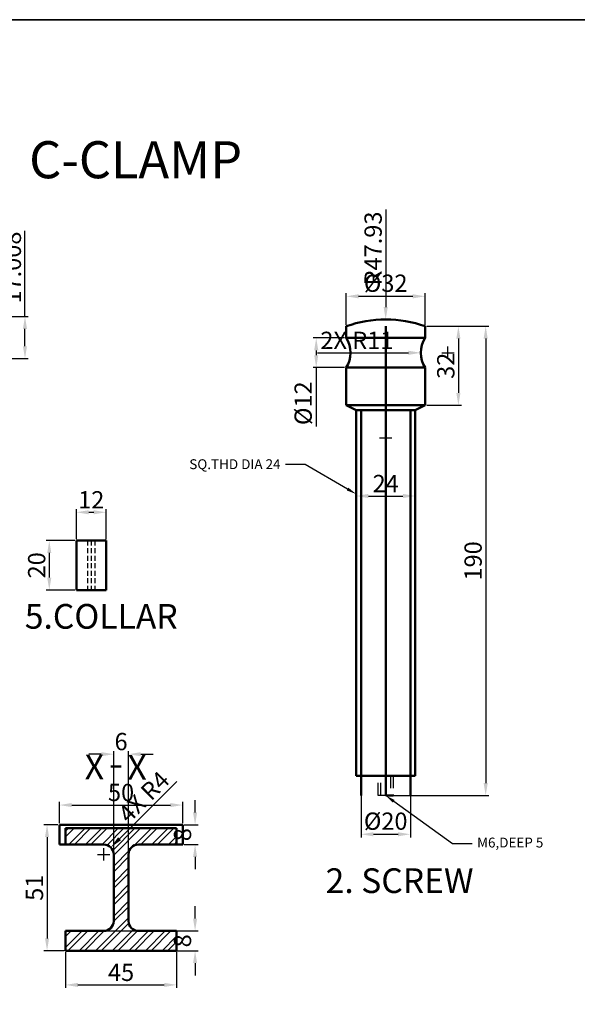
# Model space of a CAD drawing. Units: millimetres. Extents: x 210 to 1120, y -242 to 418.
# Tile 3 of 4: x 563 to 789, y 20 to 418. Entities that reach past the tile are written whole.
import ezdxf
from ezdxf import colors
from ezdxf.entities.mleader import LeaderData, LeaderLine
from ezdxf.math import Vec2, Vec3

# ---------------------------------------------------------------- set-up
doc = ezdxf.new("R2010")
doc.units = ezdxf.units.MM
doc.header["$LTSCALE"] = 0.4
doc.linetypes.add('DASHED', pattern=[19.05, 12.7, -6.35])
for name, color, linetype, lineweight in [('M-DIMS', 2, 'Continuous', 25), ('M-HATC', 8, 'Continuous', 18), ('M-HIDN', 4, 'DASHED', 25), ('M-OUTL', 7, 'Continuous', 50), ('M-TEXT', 3, 'Continuous', 25), ('M-TTLB', 7, 'Continuous', 35)]:
    doc.layers.add(name, color=color, linetype=linetype, lineweight=lineweight)
doc.styles.get("Standard").update_dxf_attribs({"font": 'arial.ttf'})
doc.dimstyles.new('ISO-25', dxfattribs={"dimtxt": 7, "dimasz": 5, "dimexe": 1.25, "dimexo": 0.625, "dimtad": 1, "dimtxsty": 'Standard', "dimcen": 2.5, "dimadec": 0, "dimazin": 0, "dimtfac": 1, "dimtofl": 0, "dimtmove": 0, "dimatfit": 3, "dimfxl": 1, "dimarcsym": 0})

# ---------------------------------------------------------------- blocks, each defined once
blk = doc.blocks.new('*D18')
at = {"layer": 'Defpoints', "color": 0, "transparency": 16777216}
for p in [(581.44, 41.35), (626.44, 41.35), (626.44, 27.51)]:
    blk.add_point(p, dxfattribs=at)
at = {"layer": 'M-DIMS', "color": 0, "lineweight": -2, "transparency": 16777216}
for p, q in [((581.44, 40.72), (581.44, 26.26)), ((626.44, 40.72), (626.44, 26.26)), ((586.44, 27.51), (621.44, 27.51))]:
    blk.add_line(p, q, dxfattribs=at)
at = {"layer": 'M-DIMS', "color": 0, "transparency": 16777216}
for points in [[(586.44, 28.34), (586.44, 26.67), (581.44, 27.51)], [(621.44, 28.34), (621.44, 26.67), (626.44, 27.51)]]:
    blk.add_solid(points, dxfattribs=at)
at = {"layer": 'M-DIMS', "color": 0, "transparency": 16777216, "insert": (603.94, 31.69), "char_height": 7, "attachment_point": 5}
blk.add_mtext('45', dxfattribs=at)
blk = doc.blocks.new('*D19')
at = {"layer": 'Defpoints', "color": 0, "transparency": 16777216}
for p in [(628.94, 100.33), (578.94, 92.35), (628.94, 92.35)]:
    blk.add_point(p, dxfattribs=at)
at = {"layer": 'M-DIMS', "color": 0, "lineweight": -2, "transparency": 16777216}
for p, q in [((578.94, 92.97), (578.94, 101.58)), ((583.94, 100.33), (623.94, 100.33)), ((628.94, 92.97), (628.94, 101.58))]:
    blk.add_line(p, q, dxfattribs=at)
at = {"layer": 'M-DIMS', "color": 0, "transparency": 16777216}
for points in [[(583.94, 101.17), (583.94, 99.5), (578.94, 100.33)], [(623.94, 101.17), (623.94, 99.5), (628.94, 100.33)]]:
    blk.add_solid(points, dxfattribs=at)
at = {"layer": 'M-DIMS', "color": 0, "transparency": 16777216, "insert": (603.94, 104.53), "char_height": 7, "attachment_point": 5}
blk.add_mtext('50', dxfattribs=at)
blk = doc.blocks.new('*D21')
at = {"layer": 'Defpoints', "color": 0, "transparency": 16777216}
for p in [(727.19, 306.33), (695.19, 294.2), (727.19, 294.2)]:
    blk.add_point(p, dxfattribs=at)
at = {"layer": 'M-DIMS', "color": 0, "lineweight": -2, "transparency": 16777216}
for p, q in [((695.19, 294.83), (695.19, 307.58)), ((727.19, 294.83), (727.19, 307.58)), ((700.19, 306.33), (722.19, 306.33))]:
    blk.add_line(p, q, dxfattribs=at)
at = {"layer": 'M-DIMS', "color": 0, "transparency": 16777216}
for points in [[(700.19, 307.17), (700.19, 305.5), (695.19, 306.33)], [(722.19, 307.17), (722.19, 305.5), (727.19, 306.33)]]:
    blk.add_solid(points, dxfattribs=at)
at = {"layer": 'M-DIMS', "color": 0, "transparency": 16777216, "insert": (711.19, 310.73), "char_height": 7, "attachment_point": 5}
blk.add_mtext('%%C32', dxfattribs=at)
blk = doc.blocks.new('*D22')
at = {"layer": 'Defpoints', "color": 0, "transparency": 16777216}
for p in [(695.19, 289.46), (683.04, 277.46), (695.19, 277.46)]:
    blk.add_point(p, dxfattribs=at)
at = {"layer": 'M-DIMS', "color": 0, "lineweight": -2, "transparency": 16777216}
for p, q in [((694.56, 289.46), (681.79, 289.46)), ((683.04, 284.46), (683.04, 282.46)), ((694.56, 277.46), (681.79, 277.46)), ((683.04, 277.46), (683.04, 253.64))]:
    blk.add_line(p, q, dxfattribs=at)
at = {"layer": 'M-DIMS', "color": 0, "transparency": 16777216}
for points in [[(682.21, 284.46), (683.88, 284.46), (683.04, 289.46)], [(682.21, 282.46), (683.88, 282.46), (683.04, 277.46)]]:
    blk.add_solid(points, dxfattribs=at)
at = {"layer": 'M-DIMS', "color": 0, "transparency": 16777216, "insert": (678.65, 263.05), "char_height": 7, "attachment_point": 5, "rotation": 90}
blk.add_mtext('%%C12', dxfattribs=at)
blk = doc.blocks.new('*D23')
at = {"layer": 'Defpoints', "color": 0, "transparency": 16777216}
for p in [(727.19, 294.2), (727.19, 262.2), (740.65, 262.2)]:
    blk.add_point(p, dxfattribs=at)
at = {"layer": 'M-DIMS', "color": 0, "lineweight": -2, "transparency": 16777216}
for p, q in [((727.81, 294.2), (741.9, 294.2)), ((740.65, 289.2), (740.65, 267.2)), ((727.81, 262.2), (741.9, 262.2))]:
    blk.add_line(p, q, dxfattribs=at)
at = {"layer": 'M-DIMS', "color": 0, "transparency": 16777216}
for points in [[(739.82, 289.2), (741.48, 289.2), (740.65, 294.2)], [(739.82, 267.2), (741.48, 267.2), (740.65, 262.2)]]:
    blk.add_solid(points, dxfattribs=at)
at = {"layer": 'M-DIMS', "color": 0, "transparency": 16777216, "insert": (736.45, 278.2), "char_height": 7, "attachment_point": 5, "rotation": 90}
blk.add_mtext('32', dxfattribs=at)
blk = doc.blocks.new('*D24')
at = {"layer": 'Defpoints', "color": 0, "transparency": 16777216}
for p in [(701.19, 112.2), (721.19, 112.2), (721.19, 88.5)]:
    blk.add_point(p, dxfattribs=at)
at = {"layer": 'M-DIMS', "color": 0, "lineweight": -2, "transparency": 16777216}
for p, q in [((701.19, 111.58), (701.19, 87.25)), ((721.19, 111.58), (721.19, 87.25)), ((706.19, 88.5), (716.19, 88.5))]:
    blk.add_line(p, q, dxfattribs=at)
at = {"layer": 'M-DIMS', "color": 0, "transparency": 16777216}
for points in [[(706.19, 89.33), (706.19, 87.67), (701.19, 88.5)], [(716.19, 89.33), (716.19, 87.67), (721.19, 88.5)]]:
    blk.add_solid(points, dxfattribs=at)
at = {"layer": 'M-DIMS', "color": 0, "transparency": 16777216, "insert": (711.19, 92.9), "char_height": 7, "attachment_point": 5}
blk.add_mtext('%%C20', dxfattribs=at)
blk = doc.blocks.new('*D25')
at = {"layer": 'Defpoints', "color": 0, "ltscale": 0.4, "transparency": 16777216}
for p in [(699.19, 228.99), (723.19, 228.99), (723.19, 225.47)]:
    blk.add_point(p, dxfattribs=at)
at = {"layer": 'M-DIMS', "color": 0, "lineweight": -2, "ltscale": 0.4, "transparency": 16777216}
for p, q in [((699.19, 228.37), (699.19, 224.22)), ((723.19, 228.37), (723.19, 224.22)), ((704.19, 225.47), (718.19, 225.47))]:
    blk.add_line(p, q, dxfattribs=at)
at = {"layer": 'M-DIMS', "color": 0, "ltscale": 0.4, "transparency": 16777216}
for points in [[(704.19, 226.31), (704.19, 224.64), (699.19, 225.47)], [(718.19, 226.31), (718.19, 224.64), (723.19, 225.47)]]:
    blk.add_solid(points, dxfattribs=at)
at = {"layer": 'M-DIMS', "color": 0, "ltscale": 0.4, "transparency": 16777216, "insert": (711.19, 229.61), "char_height": 7, "attachment_point": 5}
blk.add_mtext('24', dxfattribs=at)
blk = doc.blocks.new('*D33')
at = {"layer": 'Defpoints', "color": 0, "ltscale": 0.4, "transparency": 16777216}
for p in [(727.19, 294.2), (711.19, 104.2), (751.72, 104.2)]:
    blk.add_point(p, dxfattribs=at)
at = {"layer": 'M-DIMS', "color": 0, "lineweight": -2, "ltscale": 0.4, "transparency": 16777216}
for p, q in [((727.81, 294.2), (752.97, 294.2)), ((751.72, 289.2), (751.72, 109.2)), ((711.81, 104.2), (752.97, 104.2))]:
    blk.add_line(p, q, dxfattribs=at)
at = {"layer": 'M-DIMS', "color": 0, "ltscale": 0.4, "transparency": 16777216}
for points in [[(750.88, 289.2), (752.55, 289.2), (751.72, 294.2)], [(750.88, 109.2), (752.55, 109.2), (751.72, 104.2)]]:
    blk.add_solid(points, dxfattribs=at)
at = {"layer": 'M-DIMS', "color": 0, "ltscale": 0.4, "transparency": 16777216, "insert": (747.52, 199.2), "char_height": 7, "attachment_point": 5, "rotation": 90}
blk.add_mtext('190', dxfattribs=at)
blk = doc.blocks.new('*D41')
at = {"layer": 'Defpoints', "color": 0, "ltscale": 0.4, "transparency": 16777216}
for p in [(597.86, 218.89), (585.86, 207.41), (597.86, 207.41)]:
    blk.add_point(p, dxfattribs=at)
at = {"layer": 'M-DIMS', "color": 0, "lineweight": -2, "ltscale": 0.4, "transparency": 16777216}
for p, q in [((585.86, 208.03), (585.86, 220.14)), ((597.86, 208.03), (597.86, 220.14)), ((590.86, 218.89), (592.86, 218.89))]:
    blk.add_line(p, q, dxfattribs=at)
at = {"layer": 'M-DIMS', "color": 0, "ltscale": 0.4, "transparency": 16777216}
for points in [[(590.86, 219.72), (590.86, 218.05), (585.86, 218.89)], [(592.86, 219.72), (592.86, 218.05), (597.86, 218.89)]]:
    blk.add_solid(points, dxfattribs=at)
at = {"layer": 'M-DIMS', "color": 0, "ltscale": 0.4, "transparency": 16777216, "insert": (591.86, 223.03), "char_height": 7, "attachment_point": 5}
blk.add_mtext('12', dxfattribs=at)
blk = doc.blocks.new('*D42')
at = {"layer": 'Defpoints', "color": 0, "ltscale": 0.4, "transparency": 16777216}
for p in [(585.86, 207.41), (574.84, 187.41), (585.86, 187.41)]:
    blk.add_point(p, dxfattribs=at)
at = {"layer": 'M-DIMS', "color": 0, "lineweight": -2, "ltscale": 0.4, "transparency": 16777216}
for p, q in [((585.24, 207.41), (573.59, 207.41)), ((574.84, 202.41), (574.84, 192.41)), ((585.24, 187.41), (573.59, 187.41))]:
    blk.add_line(p, q, dxfattribs=at)
at = {"layer": 'M-DIMS', "color": 0, "ltscale": 0.4, "transparency": 16777216}
for points in [[(574.01, 202.41), (575.67, 202.41), (574.84, 207.41)], [(574.01, 192.41), (575.67, 192.41), (574.84, 187.41)]]:
    blk.add_solid(points, dxfattribs=at)
at = {"layer": 'M-DIMS', "color": 0, "ltscale": 0.4, "transparency": 16777216, "insert": (570.64, 197.41), "char_height": 7, "attachment_point": 5, "rotation": 90}
blk.add_mtext('20', dxfattribs=at)
blk = doc.blocks.new('*D48')
at = {"layer": 'Defpoints', "color": 0, "ltscale": 0.4, "transparency": 16777216}
for p in [(342.72, 298.14), (565, 298.14), (432.22, 281.13)]:
    blk.add_point(p, dxfattribs=at)
at = {"layer": 'M-DIMS', "color": 0, "lineweight": -2, "ltscale": 0.4, "transparency": 16777216}
for p, q in [((565, 298.14), (565, 332.81)), ((343.34, 298.14), (566.25, 298.14)), ((565, 286.13), (565, 293.14)), ((432.84, 281.13), (566.25, 281.13))]:
    blk.add_line(p, q, dxfattribs=at)
at = {"layer": 'M-DIMS', "color": 0, "ltscale": 0.4, "transparency": 16777216}
for points in [[(564.16, 293.14), (565.83, 293.14), (565, 298.14)], [(564.16, 286.13), (565.83, 286.13), (565, 281.13)]]:
    blk.add_solid(points, dxfattribs=at)
at = {"layer": 'M-DIMS', "color": 0, "ltscale": 0.4, "transparency": 16777216, "insert": (560.8, 317.98), "char_height": 7, "attachment_point": 5, "rotation": 90}
blk.add_mtext('17.008', dxfattribs=at)
blk = doc.blocks.new('*D50')
at = {"layer": 'Defpoints', "color": 0, "ltscale": 0.4, "transparency": 16777216}
for p in [(578.94, 92.35), (573.94, 41.35), (581.44, 41.35)]:
    blk.add_point(p, dxfattribs=at)
at = {"layer": 'M-DIMS', "color": 0, "lineweight": -2, "ltscale": 0.4, "transparency": 16777216}
for p, q in [((578.32, 92.35), (572.69, 92.35)), ((573.94, 87.35), (573.94, 46.35)), ((580.82, 41.35), (572.69, 41.35))]:
    blk.add_line(p, q, dxfattribs=at)
at = {"layer": 'M-DIMS', "color": 0, "ltscale": 0.4, "transparency": 16777216}
for points in [[(573.11, 87.35), (574.77, 87.35), (573.94, 92.35)], [(573.11, 46.35), (574.77, 46.35), (573.94, 41.35)]]:
    blk.add_solid(points, dxfattribs=at)
at = {"layer": 'M-DIMS', "color": 0, "ltscale": 0.4, "transparency": 16777216, "insert": (569.74, 66.85), "char_height": 7, "attachment_point": 5, "rotation": 90}
blk.add_mtext('51', dxfattribs=at)
blk = doc.blocks.new('*D51')
at = {"layer": 'Defpoints', "color": 0, "ltscale": 0.4, "transparency": 16777216}
for p in [(581.44, 49.35), (633.94, 49.35), (581.44, 41.35)]:
    blk.add_point(p, dxfattribs=at)
at = {"layer": 'M-DIMS', "color": 0, "lineweight": -2, "ltscale": 0.4, "transparency": 16777216}
for p, q in [((633.94, 54.35), (633.94, 59.35)), ((582.07, 49.35), (635.19, 49.35)), ((582.07, 41.35), (635.19, 41.35)), ((633.94, 36.35), (633.94, 31.35))]:
    blk.add_line(p, q, dxfattribs=at)
at = {"layer": 'M-DIMS', "color": 0, "ltscale": 0.4, "transparency": 16777216}
for points in [[(633.11, 54.35), (634.77, 54.35), (633.94, 49.35)], [(633.11, 36.35), (634.77, 36.35), (633.94, 41.35)]]:
    blk.add_solid(points, dxfattribs=at)
at = {"layer": 'M-DIMS', "color": 0, "ltscale": 0.4, "transparency": 16777216, "insert": (629.74, 45.35), "char_height": 7, "attachment_point": 5, "rotation": 90}
blk.add_mtext('8', dxfattribs=at)
blk = doc.blocks.new('*D52')
at = {"layer": 'Defpoints', "color": 0, "ltscale": 0.4, "transparency": 16777216}
for p in [(628.94, 92.35), (633.94, 92.35), (628.94, 84.35)]:
    blk.add_point(p, dxfattribs=at)
at = {"layer": 'M-DIMS', "color": 0, "lineweight": -2, "ltscale": 0.4, "transparency": 16777216}
for p, q in [((633.94, 97.35), (633.94, 102.35)), ((629.57, 92.35), (635.19, 92.35)), ((629.57, 84.35), (635.19, 84.35)), ((633.94, 79.35), (633.94, 74.35))]:
    blk.add_line(p, q, dxfattribs=at)
at = {"layer": 'M-DIMS', "color": 0, "ltscale": 0.4, "transparency": 16777216}
for points in [[(633.11, 97.35), (634.77, 97.35), (633.94, 92.35)], [(633.11, 79.35), (634.77, 79.35), (633.94, 84.35)]]:
    blk.add_solid(points, dxfattribs=at)
at = {"layer": 'M-DIMS', "color": 0, "ltscale": 0.4, "transparency": 16777216, "insert": (629.74, 88.35), "char_height": 7, "attachment_point": 5, "rotation": 90}
blk.add_mtext('8', dxfattribs=at)
blk = doc.blocks.new('*D53')
at = {"layer": 'Defpoints', "color": 0, "ltscale": 0.4, "transparency": 16777216}
for p in [(606.94, 120.93), (600.94, 80.35), (606.94, 80.35)]:
    blk.add_point(p, dxfattribs=at)
at = {"layer": 'M-DIMS', "color": 0, "lineweight": -2, "ltscale": 0.4, "transparency": 16777216}
for p, q in [((595.94, 120.93), (590.94, 120.93)), ((600.94, 80.97), (600.94, 122.18)), ((606.94, 80.97), (606.94, 122.18)), ((611.94, 120.93), (616.94, 120.93))]:
    blk.add_line(p, q, dxfattribs=at)
at = {"layer": 'M-DIMS', "color": 0, "ltscale": 0.4, "transparency": 16777216}
for points in [[(595.94, 121.76), (595.94, 120.09), (600.94, 120.93)], [(611.94, 121.76), (611.94, 120.09), (606.94, 120.93)]]:
    blk.add_solid(points, dxfattribs=at)
at = {"layer": 'M-DIMS', "color": 0, "ltscale": 0.4, "transparency": 16777216, "insert": (603.94, 125.13), "char_height": 7, "attachment_point": 5}
blk.add_mtext('6', dxfattribs=at)
blk = doc.blocks.new('*D57')
at = {"layer": 'Defpoints', "color": 0, "ltscale": 0.4, "transparency": 16777216}
for p in [(596.94, 80.35), (599.77, 83.17)]:
    blk.add_point(p, dxfattribs=at)
at = {"layer": 'M-DIMS', "color": 0, "lineweight": -2, "ltscale": 0.4, "transparency": 16777216}
for p, q in [((626.56, 109.89), (603.31, 86.7)), ((594.44, 80.35), (599.44, 80.35)), ((596.94, 77.85), (596.94, 82.85))]:
    blk.add_line(p, q, dxfattribs=at)
at = {"layer": 'M-DIMS', "color": 0, "ltscale": 0.4, "transparency": 16777216}
blk.add_solid([(602.73, 87.29), (603.9, 86.11), (599.77, 83.17)], dxfattribs=at)
at = {"layer": 'M-DIMS', "color": 0, "ltscale": 0.4, "transparency": 16777216, "insert": (613.79, 102.98), "char_height": 7, "attachment_point": 5, "rotation": 44.9182}
blk.add_mtext('4X R4', dxfattribs=at)
blk = doc.blocks.new('*D58')
at = {"layer": 'Defpoints', "color": 0, "ltscale": 0.4, "transparency": 16777216}
for p in [(711.19, 296.95), (711.19, 249.02)]:
    blk.add_point(p, dxfattribs=at)
at = {"layer": 'M-DIMS', "color": 0, "lineweight": -2, "ltscale": 0.4, "transparency": 16777216}
for p, q in [((711.19, 341.49), (711.19, 301.95)), ((711.19, 246.52), (711.19, 251.52)), ((708.69, 249.02), (713.69, 249.02))]:
    blk.add_line(p, q, dxfattribs=at)
at = {"layer": 'M-DIMS', "color": 0, "ltscale": 0.4, "transparency": 16777216}
blk.add_solid([(710.36, 301.95), (712.02, 301.95), (711.19, 296.95)], dxfattribs=at)
at = {"layer": 'M-DIMS', "color": 0, "ltscale": 0.4, "transparency": 16777216, "insert": (706.99, 325.71), "char_height": 7, "attachment_point": 5, "rotation": 89.9994}
blk.add_mtext('R47.93', dxfattribs=at)
blk = doc.blocks.new('*D59')
at = {"layer": 'Defpoints', "color": 0, "ltscale": 0.4, "transparency": 16777216}
for p in [(725.41, 283.46), (736.41, 283.46)]:
    blk.add_point(p, dxfattribs=at)
at = {"layer": 'M-DIMS', "color": 0, "lineweight": -2, "ltscale": 0.4, "transparency": 16777216}
for p, q in [((683.62, 283.46), (720.41, 283.46)), ((733.91, 283.46), (738.91, 283.46)), ((736.41, 280.96), (736.41, 285.96))]:
    blk.add_line(p, q, dxfattribs=at)
at = {"layer": 'M-DIMS', "color": 0, "ltscale": 0.4, "transparency": 16777216}
blk.add_solid([(720.41, 284.29), (720.41, 282.62), (725.41, 283.46)], dxfattribs=at)
at = {"layer": 'M-DIMS', "color": 0, "ltscale": 0.4, "transparency": 16777216, "insert": (699.52, 287.6), "char_height": 7, "attachment_point": 5, "rotation": 0.0011}
blk.add_mtext('2X R11', dxfattribs=at)

msp = doc.modelspace()

# ---------------------------------------------------------------- hatches: boundary and pattern name
at = {"layer": 'M-HATC'}
h = msp.add_hatch(dxfattribs=at)
h.set_pattern_fill('ANSI32', color=256, scale=0.5)
h.paths.add_polyline_path([(626.4411, 90.9516), (581.4411, 90.9516), (581.4411, 84.349), (596.9411, 84.349, -0.41421356), (600.9411, 80.349), (600.9411, 53.349, -0.41421356), (596.9411, 49.349), (581.4411, 49.349), (581.4411, 41.349), (626.4411, 41.349), (626.4411, 49.349), (610.9411, 49.349, -0.41421356), (606.9411, 53.349), (606.9411, 80.349, -0.41421356), (610.9411, 84.349), (626.4411, 84.349)])

# ---------------------------------------------------------------- linework, layer by layer
at = {"layer": 'M-HIDN', "ltscale": 0.4}
for p, q in [((590.362, 207.4059), (590.362, 187.4059)), ((591.862, 207.4059), (591.862, 187.4059)), ((593.362, 207.4059), (593.362, 187.4059))]:
    msp.add_line(p, q, dxfattribs=at)
at = {"layer": 'M-HIDN'}
for p, q in [((708.1885, 104.2017), (708.1885, 112.2017)), ((709.1885, 104.2017), (709.1885, 112.2017)), ((713.1885, 112.2017), (713.1885, 104.2017)), ((714.1885, 112.2017), (714.1885, 104.2017)), ((711.1885, 104.2017), (708.1885, 104.2017))]:
    msp.add_line(p, q, dxfattribs=at)
at = {"layer": 'M-OUTL'}
for p, q in [((695.1885, 289.4572), (695.1885, 294.2017)), ((711.1885, 294.2017), (711.1885, 104.2017)), ((727.1885, 294.2017), (727.1885, 289.4572)), ((695.1885, 289.4572), (727.1885, 289.4572)), ((695.1885, 262.2017), (695.1885, 277.4572)), ((695.1885, 277.4572), (727.1885, 277.4572)), ((727.1885, 277.4572), (727.1885, 262.2017)), ((695.1885, 262.2017), (727.1885, 262.2017)), ((695.1885, 262.2017), (699.1885, 260.2017)), ((699.1885, 260.2017), (699.1885, 112.2017)), ((701.1885, 260.2017), (701.1885, 104.2017)), ((721.1885, 260.2017), (721.1885, 104.2017)), ((727.1885, 262.2017), (723.1885, 260.2017)), ((723.1885, 260.2017), (723.1885, 112.2017)), ((601.3631, 115.9264), (599.8342, 115.9264)), ((599.8342, 115.9264), (603.9853, 115.9264)), ((723.1885, 112.2017), (699.1885, 112.2017)), ((714.1885, 104.2017), (711.1885, 104.2017)), ((578.9411, 92.349), (628.9411, 92.349)), ((578.9411, 84.349), (578.9411, 92.349)), ((628.9411, 92.349), (628.9411, 84.349)), ((581.4411, 90.9516), (626.4411, 90.9516)), ((581.4411, 84.349), (581.4411, 90.9516)), ((626.4411, 90.9516), (626.4411, 84.349)), ((596.9411, 84.349), (578.9411, 84.349)), ((628.9411, 84.349), (610.9411, 84.349)), ((600.9411, 80.349), (600.9411, 53.349)), ((606.9411, 80.349), (606.9411, 53.349)), ((581.4411, 49.349), (596.9411, 49.349)), ((581.4411, 41.349), (581.4411, 49.349)), ((610.9411, 49.349), (626.4411, 49.349)), ((626.4411, 49.349), (626.4411, 41.349)), ((626.4411, 41.349), (581.4411, 41.349)), ((581.4411, 41.349), (626.4411, 41.349))]:
    msp.add_line(p, q, dxfattribs=at)
at = {"layer": 'M-OUTL', "ltscale": 0.4}
for p, q in [((699.1885, 260.2017), (723.1885, 260.2017)), ((585.862, 207.4059), (597.862, 207.4059)), ((585.862, 187.4059), (585.862, 207.4059)), ((597.862, 207.4059), (597.862, 187.4059)), ((597.862, 187.4059), (585.862, 187.4059))]:
    msp.add_line(p, q, dxfattribs=at)
at = {"layer": 'M-OUTL'}
for centre, radius, start, end in [((711.1885, 249.0204), 47.9307, 70.499481, 109.500519), ((685.9696, 283.4572), 10.9994, 326.942366, 33.057634), ((736.4074, 283.4572), 10.9994, 146.942366, 213.057634), ((596.9411, 80.349), 4, 0, 90), ((610.9411, 80.349), 4, 90, 180), ((596.9411, 53.349), 4, 270, 0), ((610.9411, 53.349), 4, 180, 270)]:
    msp.add_arc(centre, radius, start, end, dxfattribs=at)
at = {"layer": 'M-TTLB', "ltscale": 0.4}
msp.add_lwpolyline([(210.1659, 418.3486), (1119.5264, 418.3486), (1119.5264, -242.3444), (210.1659, -242.3444)], close=True, dxfattribs=at)

# ---------------------------------------------------------------- texts
at = {"layer": 'M-TEXT', "ltscale": 0.4, "insert": (452.2266, 369.1481), "char_height": 15, "attachment_point": 1}
msp.add_mtext_dynamic_manual_height_columns('\\pxqc; C-CLAMP', width=310.631866, gutter_width=12.5, heights=[0], dxfattribs=at)
at = {"layer": 'M-TEXT', "attachment_point": 1}
for s, width, insert, char_height in [('\\pxqc;{\\H0.66667x;5.COLLAR} ', 102.502816, (544.6548, 181.7422), 15), ('X', 4.451993, (589.2112, 120.7711), 10), ('X', 4.451993, (606.5122, 120.6317), 10), ('\\pxqc;{\\H0.66667x;2. SCREW} ', 102.831898, (665.4087, 74.7214), 15)]:
    msp.add_mtext_dynamic_manual_height_columns(s, width=width, gutter_width=12.5, heights=[0], dxfattribs=dict(at, insert=insert, char_height=char_height))

# ---------------------------------------------------------------- dimensions: what is measured, and where the dimension line sits
at = {"layer": 'M-DIMS', "ltscale": 0.4}
dim = msp.add_radius_dim(center=(711.1885, 249.0204), mpoint=(711.189, 296.951), dimstyle='ISO-25', override={"dimdec": 2, "dimlfac": 1, "dimrnd": 0, "dimzin": 0, "dimdsep": 46, "dimlunit": 2}, dxfattribs=at)
dim.commit()
dim.dimension.update_dxf_attribs({"geometry": '*D58', "text_midpoint": (711.1893, 325.7094), "dimtype": 164})
for base, p1, p2, override, picture, middle in [((564.9982, 298.1425), (432.2189, 281.1344), (342.7189, 298.1425), {"dimdec": 3, "dimlfac": 1, "dimrnd": 0, "dimzin": 0, "dimdsep": 46, "dimlunit": 2}, '*D48', (560.7991, 317.9752)), ((751.7164, 104.2017), (727.1885, 294.2017), (711.1885, 104.2017), {"dimclrd": 0, "dimclre": 0, "dimclrt": 0}, '*D33', (747.5174, 199.2017)), ((574.8398, 187.4059), (585.862, 207.4059), (585.862, 187.4059), {"dimclrd": 0, "dimclre": 0, "dimclrt": 0}, '*D42', (570.6407, 197.4059)), ((633.9411, 92.349), (628.9411, 84.349), (628.9411, 92.349), {"dimdec": 0, "dimlfac": 1, "dimrnd": 0, "dimzin": 0, "dimdsep": 46, "dimlunit": 2}, '*D52', (629.7421, 88.349)), ((573.9411, 41.349), (578.9411, 92.349), (581.4411, 41.349), {"dimdec": 0, "dimlfac": 1, "dimrnd": 0, "dimzin": 0, "dimdsep": 46, "dimlunit": 2}, '*D50', (569.7421, 66.849)), ((633.9411, 49.349), (581.4411, 41.349), (581.4411, 49.349), {"dimdec": 0, "dimlfac": 1, "dimrnd": 0, "dimzin": 0, "dimdsep": 46, "dimlunit": 2}, '*D51', (629.7421, 45.349))]:
    dim = msp.add_linear_dim(base=base, p1=p1, p2=p2, angle=90, dimstyle='ISO-25', override=override, dxfattribs=at)
    dim.commit()
    dim.dimension.update_dxf_attribs({"geometry": picture, "text_midpoint": middle})
at = {"layer": 'M-DIMS'}
for base, p1, p2, picture, middle in [((727.1885, 306.3337), (695.1885, 294.2017), (727.1885, 294.2017), '*D21', (711.1885, 310.7285)), ((721.1885, 88.5008), (701.1885, 112.2017), (721.1885, 112.2017), '*D24', (711.1885, 92.8956))]:
    dim = msp.add_linear_dim(base=base, p1=p1, p2=p2, text='%%C<>', dimstyle='ISO-25', override={"dimclrd": 0, "dimclre": 0, "dimclrt": 0}, dxfattribs=at)
    dim.commit()
    dim.dimension.update_dxf_attribs({"geometry": picture, "text_midpoint": middle})
at = {"layer": 'M-DIMS', "ltscale": 0.4}
for center, mpoint, text, picture, middle in [((736.4074, 283.4572), (725.4079, 283.457), '2X <>', '*D59', (699.5151, 287.5982)), ((596.9411, 80.349), (599.7736, 83.1734), '4X <>', '*D57', (613.7945, 102.983))]:
    dim = msp.add_radius_dim(center=center, mpoint=mpoint, text=text, dimstyle='ISO-25', override={"dimdec": 0, "dimlfac": 1, "dimrnd": 0, "dimzin": 0, "dimdsep": 46, "dimlunit": 2}, dxfattribs=at)
    dim.commit()
    dim.dimension.update_dxf_attribs({"geometry": picture, "text_midpoint": middle})
at = {"layer": 'M-DIMS'}
dim = msp.add_linear_dim(base=(740.6513, 262.2017), p1=(727.1885, 294.2017), p2=(727.1885, 262.2017), angle=90, dimstyle='ISO-25', override={"dimclrd": 0, "dimclre": 0, "dimclrt": 0}, dxfattribs=at)
dim.commit()
dim.dimension.update_dxf_attribs({"geometry": '*D23', "text_midpoint": (736.4499, 278.2017)})
dim = msp.add_linear_dim(base=(683.0418, 277.4572), p1=(695.1885, 289.4572), p2=(695.1885, 277.4572), angle=90, text='%%C<>', dimstyle='ISO-25', override={"dimclrd": 0, "dimclre": 0, "dimclrt": 0}, dxfattribs=at)
dim.commit()
dim.dimension.update_dxf_attribs({"geometry": '*D22', "text_midpoint": (678.647, 263.0464)})
at = {"layer": 'M-DIMS', "ltscale": 0.4}
for base, p1, p2, override, picture, middle in [((723.1885, 225.4725), (699.1885, 228.9917), (723.1885, 228.9917), {"dimclrd": 0, "dimclre": 0, "dimclrt": 0}, '*D25', (711.1885, 229.6118)), ((597.862, 218.8863), (585.862, 207.4059), (597.862, 207.4059), {"dimclrd": 0, "dimclre": 0, "dimclrt": 0}, '*D41', (591.862, 223.0256)), ((606.9411, 120.9264), (600.9411, 80.349), (606.9411, 80.349), {"dimdec": 0, "dimlfac": 1, "dimrnd": 0, "dimzin": 0, "dimdsep": 46, "dimlunit": 2}, '*D53', (603.9411, 125.1254))]:
    dim = msp.add_linear_dim(base=base, p1=p1, p2=p2, dimstyle='ISO-25', override=override, dxfattribs=at)
    dim.commit()
    dim.dimension.update_dxf_attribs({"geometry": picture, "text_midpoint": middle})
at = {"layer": 'M-DIMS'}
dim = msp.add_linear_dim(base=(628.9411, 100.335), p1=(578.9411, 92.349), p2=(628.9411, 92.349), dimstyle='ISO-25', override={"dimclrd": 0, "dimclre": 0, "dimclrt": 0}, dxfattribs=at)
dim.commit()
dim.dimension.update_dxf_attribs({"geometry": '*D19', "text_midpoint": (603.9411, 100.335), "dimtype": 160})
dim = msp.add_linear_dim(base=(626.4411, 27.5068), p1=(581.4411, 41.349), p2=(626.4411, 41.349), dimstyle='ISO-25', override={"dimclrd": 0, "dimclre": 0, "dimclrt": 0}, dxfattribs=at)
dim.commit()
dim.dimension.update_dxf_attribs({"geometry": '*D18', "text_midpoint": (603.9411, 31.6915)})

# ---------------------------------------------------------------- leaders
at = {"layer": 'M-TEXT', "ltscale": 0.4}
ml = msp.add_multileader_mtext('Standard', dxfattribs=at)
ml.set_content('SQ.THD DIA 24', color=256)
ml.set_leader_properties()
ml.build(insert=Vec2(0, 0))
ctx = ml.context
ctx.base_point, ctx.plane_origin = Vec3(627.3456, 238.1983), Vec3(699.1885, 226.2946)
ctx.text_align_type = 2
notes = []
notes.append((ctx, [(0, (1, 1, 0), (678.5707, 238.1983), (-1, 0), 8, [(0, [(699.1885, 226.2946)], 0, [])])]))
ctx.mtext.insert, ctx.mtext.alignment, ctx.mtext.flow_direction = Vec3(668.5707, 240.3538), 3, 5
at = {"layer": 'M-TEXT'}
ml = msp.add_multileader_mtext('Standard', dxfattribs=at)
ml.set_content('M6,DEEP 5', color=256)
ml.set_leader_properties()
ml.build(insert=Vec2(0, 0))
ctx = ml.context
ctx.base_point, ctx.plane_origin = Vec3(746.2287, 84.7508), Vec3(711.1885, 104.2017)
notes.append((ctx, [(0, (1, 1, 0), (738.2287, 84.7508), (1, 0), 8, [(0, [(711.1885, 104.2017)], 0, [])])]))
ctx.mtext.insert, ctx.mtext.flow_direction = Vec3(748.2287, 87.1465), 5
for ctx, leaders in notes:
    for number, flags, end, landing, length, lines in leaders:
        leader = LeaderData()
        leader.index, (leader.has_last_leader_line, leader.has_dogleg_vector, leader.attachment_direction) = number, flags
        leader.last_leader_point, leader.dogleg_vector, leader.dogleg_length = Vec3(end), Vec3(landing), length
        for number, points, colour, breaks in lines:
            line = LeaderLine()
            line.index, line.vertices, line.color, line.breaks = number, Vec3.list(points), colors.encode_raw_color(colour), breaks
            leader.lines.append(line)
        ctx.leaders.append(leader)

doc.saveas('drawing.dxf')
